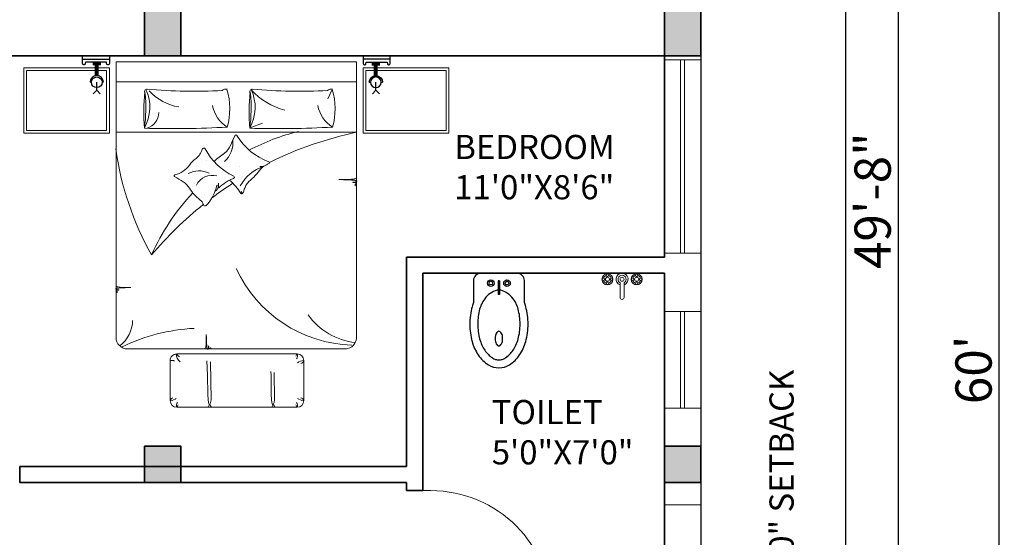
# Model space of a CAD drawing. Units: inches. Extents: x 3321 to 5237, y 11 to 1752.
# Tile 21 of 43: x 4296 to 4541, y 1306 to 1434. Entities that reach past the tile are written whole.
import ezdxf

# ---------------------------------------------------------------- set-up
doc = ezdxf.new("R2010")
doc.units = ezdxf.units.IN
for name, color, linetype, lineweight in [('A-ANNO-DIMS', 2, 'Continuous', 18), ('A-ANNO-TEXT', 7, 'Continuous', 18), ('A-AREA-IDEN', 7, 'Continuous', 18), ('A-COLS', 1, 'Continuous', 35), ('A-DOOR', 4, 'Continuous', 18), ('A-FLOR-EDGE', 7, 'Continuous', 25), ('A-GLAZ', 5, 'Continuous', 18), ('A-WALL', 7, 'Continuous', 35), ('C-PROP', 7, 'Continuous', 30), ('FUR', 42, 'Continuous', 18), ('Сантехника', 7, 'Continuous', 18)]:
    doc.layers.add(name, color=color, linetype=linetype, lineweight=lineweight)
for name, color, linetype in [('CEIL', 4, 'Continuous'), ('ELEC', 4, 'Continuous'), ('SANTEH', 7, 'Continuous'), ('wood', 26, 'Continuous')]:
    doc.layers.add(name, color=color, linetype=linetype)
doc.styles.get("Standard").update_dxf_attribs({"font": 'arial.ttf'})
doc.dimstyles.new('ISO-25', dxfattribs={"dimtxt": 9, "dimasz": 2.5, "dimexe": 1.25, "dimexo": 0.625, "dimtad": 1, "dimdec": 1, "dimlunit": 3, "dimtxsty": 'Standard', "dimcen": 2.5, "dimclrd": 4, "dimclre": 4, "dimclrt": 256, "dimadec": 0, "dimazin": 0, "dimtfac": 1, "dimtdec": 1, "dimtmove": 0, "dimatfit": 3, "dimfxl": 1, "dimarcsym": 0})

# ---------------------------------------------------------------- blocks, each defined once
blk = doc.blocks.new('*U5')
for p, q in [((0, 0), (0, -6)), ((-30, 0), (-30, -6))]:
    blk.add_line(p, q)
blk.add_lwpolyline([(0, 0), (0, 30), (-1.75, 30), (-1.75, 0)], close=True)
blk.add_arc((0, 0), 30, 90, 180)
blk = doc.blocks.new('*D61')
at = {"layer": 'A-ANNO-DIMS', "color": 0, "lineweight": -2, "transparency": 16777216}
for p, q in [((4502.01, 1687.34), (4515.69, 1687.34)), ((4514.44, 1093.84), (4514.44, 1684.84)), ((4502.01, 1091.34), (4515.69, 1091.34))]:
    blk.add_line(p, q, dxfattribs=at)
at = {"layer": 'A-ANNO-DIMS', "color": 0, "transparency": 16777216}
for points in [[(4514.03, 1684.84), (4514.86, 1684.84), (4514.44, 1687.34)], [(4514.03, 1093.84), (4514.86, 1093.84), (4514.44, 1091.34)]]:
    blk.add_solid(points, dxfattribs=at)
at = {"layer": 'Defpoints', "color": 0, "transparency": 16777216}
for p in [(4501.39, 1687.34), (4514.44, 1687.34), (4501.39, 1091.34)]:
    blk.add_point(p, dxfattribs=at)
at = {"layer": 'A-ANNO-DIMS', "color": 0, "transparency": 16777216, "insert": (4509.22, 1389.34), "char_height": 9, "attachment_point": 5, "rotation": 90}
blk.add_mtext('49\'-8"', dxfattribs=at)
blk = doc.blocks.new('*D64')
at = {"layer": 'A-ANNO-DIMS', "color": 0, "lineweight": -2, "transparency": 16777216}
for p, q in [((4502.01, 1707.34), (4540.73, 1707.34)), ((4539.48, 989.84), (4539.48, 1704.84)), ((4502.01, 987.34), (4540.73, 987.34))]:
    blk.add_line(p, q, dxfattribs=at)
at = {"layer": 'A-ANNO-DIMS', "color": 0, "transparency": 16777216}
for points in [[(4539.06, 1704.84), (4539.9, 1704.84), (4539.48, 1707.34)], [(4539.06, 989.84), (4539.9, 989.84), (4539.48, 987.34)]]:
    blk.add_solid(points, dxfattribs=at)
at = {"layer": 'Defpoints', "color": 0, "transparency": 16777216}
for p in [(4501.39, 1707.34), (4539.48, 1707.34), (4501.39, 987.34)]:
    blk.add_point(p, dxfattribs=at)
at = {"layer": 'A-ANNO-DIMS', "color": 0, "transparency": 16777216, "insert": (4534.26, 1347.34), "char_height": 9, "attachment_point": 5, "rotation": 90}
blk.add_mtext("60'", dxfattribs=at)
blk = doc.blocks.new('*X127')
at = {"color": 0}
for p, q in [((3155.9, 8182.9), (3155.9, 8182.9)), ((3147.8, 8143.4), (3147.8, 8143.4)), ((3283, 8049.6), (3283, 8049.6)), ((3209.5, 8023.9), (3209.5, 8023.9)), ((3251.6, 7997), (3251.6, 7997)), ((3154.1, 7950.7), (3154.1, 7950.7))]:
    blk.add_line(p, q, dxfattribs=at)
blk = doc.blocks.new('*X126')
at = {"color": 0}
for p, q in [((3155.9, 8182.9), (3155.9, 8182.9)), ((3139.8, 7939.7), (3139.8, 7939.7))]:
    blk.add_line(p, q, dxfattribs=at)
blk = doc.blocks.new('*X125')
at = {"color": 0}
for p, q in [((3155.9, 8182.9), (3155.9, 8182.9)), ((3139.8, 7939.7), (3139.8, 7939.7))]:
    blk.add_line(p, q, dxfattribs=at)
blk = doc.blocks.new('*X124')
at = {"color": 0}
for p, q in [((3163, 7776.2), (3163, 7776.2)), ((3422.2, 7761.3), (3422.2, 7761.3)), ((3236.2, 7675.7), (3236.2, 7675.7)), ((3244.3, 7698.6), (3244.3, 7698.6)), ((3340.3, 7689.4), (3340.3, 7689.4))]:
    blk.add_line(p, q, dxfattribs=at)
blk = doc.blocks.new('BED1')
for p, q in [((0, -1000), (0, 800)), ((150, 800), (0, 800)), ((150, 800), (150, -1000)), ((2058.7, 800), (150, 800)), ((528, 800), (528, -1000)), ((211.8, 614.9), (277.5, 585.4)), ((2537.2, 404.9), (2237.2, 404.9)), ((2187.2, 354.9), (2187.2, -545.1)), ((2587.2, -545.1), (2587.2, 354.9)), ((2566.3, 178.5), (2565.2, 177.4)), ((2582, 188.1), (2565.4, 174.8)), ((2565.4, 174.8), (2585.7, 165.4)), ((2582, -287.1), (2565.4, -300.5)), ((2566.3, -296.8), (2565.2, -297.9)), ((2565.4, -300.5), (2585.7, -309.9)), ((2237.2, -595.1), (2537.2, -595.1)), ((150, -1000), (0, -1000)), ((150, -1000), (2063.5, -1000))]:
    blk.add_line(p, q)
for points in [[(934, 797.9), (930.9, 797.7), (928.3, 797.4), (926.3, 796.9), (924.9, 796.3), (923.8, 795.6), (923.1, 794.8), (922.7, 793.8), (922.5, 792.7), (922.4, 791.5), (922.5, 790.3), (922.6, 789.2), (922.6, 788.3), (922.6, 787.6), (922.4, 787.3), (922, 787.4), (921.4, 787.9), (920.6, 788.9), (919.5, 790.2), (918.4, 791.6), (917.1, 793.1), (915.9, 794.6), (914.6, 796), (913.3, 797.1), (912.2, 797.9), (911.1, 798.3), (910.1, 798.4), (909.2, 798), (908.3, 797.1), (907.5, 795.8), (906.8, 793.9), (906, 791.4), (905.4, 788.5), (904.8, 785.2), (904.2, 781.7), (903.7, 778.4), (903.2, 775.4), (902.8, 772.9), (902.5, 771.3), (902.3, 770.6), (902.1, 771.2), (902, 772.8), (901.8, 775.2), (901.7, 778.1), (901.5, 781.5), (901.2, 785), (900.8, 788.4), (900.2, 791.5), (899.5, 794.1), (898.6, 796.2), (897.6, 797.9), (896.5, 799.2), (895.3, 800), (894.1, 800.5), (893, 800.7), (891.9, 800.5), (890.9, 800.1), (890, 799), (889.1, 797.1), (888.3, 794), (887.6, 789.3), (886.9, 782.9), (886.2, 774.2), (885.5, 763.1), (884.8, 749.5), (884.2, 734.2), (883.6, 718.3), (883, 702.8), (882.5, 688.8), (882, 677.5), (881.7, 669.8), (881.5, 666.9), (881.3, 669.4), (881.3, 676.7), (881.3, 687.8), (881.2, 701.5), (881.1, 716.8), (880.8, 732.6), (880.2, 748), (879.4, 761.8), (878.3, 773.2), (876.9, 782.2), (875.1, 789.2), (872.9, 794.4), (870.3, 798), (869, 799)], [(2150, -913.5), (2150, 723.2)], [(2327.6, 182.3), (2530, 185.9), (2550.8, 181.9), (2561.7, 179), (2566, 176.7), (2566.9, 174.4), (2566.3, 171.9), (2562, 169.2), (2550.3, 166.5), (2527.7, 163.9), (2490.6, 161.8), (2345.5, 160.2), (2317.8, 158.5)], [(494.7, 3.1), (458.9, 95.3)], [(2149.7, -259.9), (2150, -268.4), (2150.1, -274.1), (2150.1, -278.1), (2150, -281.4), (2149.8, -284), (2149.5, -286.1), (2149.1, -287.8), (2148.7, -289), (2148.1, -289.9), (2147.4, -290.5), (2146.6, -290.8), (2145.6, -291), (2144.6, -291), (2143.6, -291), (2142.7, -290.9), (2141.9, -290.9), (2141.4, -290.9), (2141.1, -291), (2141.2, -291.4), (2141.7, -291.9), (2142.5, -292.6), (2143.5, -293.4), (2144.7, -294.4), (2146, -295.4), (2147.2, -296.5), (2148.4, -297.6), (2149.3, -298.6), (2150, -299.6), (2150.3, -300.5), (2150.4, -301.3), (2150, -302.1), (2149.3, -302.8), (2148.2, -303.5), (2146.6, -304.1), (2144.6, -304.7), (2142.1, -305.2), (2139.3, -305.7), (2136.5, -306.2), (2133.7, -306.6), (2131.2, -307), (2129.2, -307.3), (2127.8, -307.6), (2127.3, -307.8), (2127.7, -308), (2129, -308.1), (2131, -308.2), (2133.5, -308.3), (2136.3, -308.5), (2139.2, -308.7), (2142, -309), (2144.6, -309.5), (2146.8, -310.1), (2148.6, -310.9), (2150, -311.7), (2151, -312.7), (2151.7, -313.6), (2152.1, -314.6), (2152.3, -315.6), (2152.2, -316.5), (2151.8, -317.3), (2150.9, -318.1), (2149.3, -318.8), (2146.7, -319.4), (2142.8, -320), (2137.4, -320.6), (2130.2, -321.2), (2121, -321.8), (2109.7, -322.3), (2096.9, -322.9), (2083.6, -323.4), (2070.7, -323.9), (2059.1, -324.3), (2049.6, -324.7), (2043.2, -325), (2040.8, -325.2), (2042.9, -325.3), (2049, -325.3), (2058.2, -325.3), (2069.6, -325.4), (2082.3, -325.5), (2095.6, -325.8), (2108.4, -326.2), (2119.9, -326.8), (2129.4, -327.8), (2136.9, -329), (2142.7, -330.5), (2147, -332.3), (2150, -334.4), (2150.9, -335.6)], [(2246.5, -294.4), (2530, -289.4), (2550.8, -293.4), (2561.7, -296.3), (2566, -298.6), (2566.9, -300.8), (2566.3, -303.4), (2562, -306.1), (2550.3, -308.8), (2527.7, -311.3), (2490.6, -313.5), (2345.5, -315), (2238.6, -321.8)], [(1733.7, -998.3), (1731.1, -998.1), (1729, -997.8), (1727.4, -997.4), (1726.1, -997), (1725.2, -996.4), (1724.7, -995.7), (1724.3, -994.8), (1724.1, -993.9), (1724.1, -992.9), (1724.1, -991.9), (1724.2, -991), (1724.2, -990.2), (1724.2, -989.7), (1724.1, -989.4), (1723.8, -989.5), (1723.2, -990), (1722.5, -990.8), (1721.7, -991.8), (1720.7, -993), (1719.7, -994.3), (1718.6, -995.5), (1717.5, -996.6), (1716.5, -997.6), (1715.5, -998.3), (1714.6, -998.6), (1713.8, -998.6), (1713, -998.3), (1712.3, -997.6), (1711.7, -996.5), (1711, -994.9), (1710.4, -992.9), (1709.9, -990.4), (1709.4, -987.6), (1708.9, -984.8), (1708.5, -982), (1708.1, -979.5), (1707.8, -977.4), (1707.5, -976.1), (1707.3, -975.5), (1707.1, -976), (1707, -977.3), (1706.9, -979.3), (1706.8, -981.8), (1706.7, -984.6), (1706.4, -987.5), (1706.1, -990.3), (1705.6, -992.9), (1705, -995.1), (1704.2, -996.9), (1703.4, -998.3), (1702.4, -999.3), (1701.5, -1000), (1700.5, -1000.4), (1699.6, -1000.6), (1698.7, -1000.4), (1697.8, -1000.1), (1697, -999.2), (1696.3, -997.6), (1695.7, -995), (1695.1, -991.1), (1694.5, -985.7), (1693.9, -978.5), (1693.3, -969.3), (1692.8, -957.9), (1692.2, -945.2), (1691.7, -931.9), (1691.2, -919), (1690.8, -907.4), (1690.4, -897.9), (1690.1, -891.5), (1689.9, -889.1), (1689.8, -891.2), (1689.8, -897.3), (1689.8, -906.5), (1689.7, -917.9), (1689.6, -930.6), (1689.4, -943.8), (1688.9, -956.6), (1688.3, -968.1), (1687.3, -977.6), (1686.1, -985.2), (1684.6, -991), (1682.8, -995.3), (1680.7, -998.3), (1679.6, -999.2)]]:
    blk.add_lwpolyline(points)
for points in [[(205.5, 619.6, 0.267769), (215.1, 582.4, -0.037739), (204.3, 21.8, 0.684696), (236.7, 5.5, -0.060702), (497.2, 0.1, -0.046649), (225.9, 3.1, -1.318436)], [(489.2, 619.6, 0.144019), (207.6, 617.9, 0.248643)], [(497.2, 0.1, 0.021276), (489.2, 619.6, -0.206383), (326.6, 509.4, 0.237198)], [(211.8, 12.8, 0.143972), (361.6, 262.9, 1.292232)], [(886.4, -150, -0.069098), (985, -66.5, 0.658965), (982.1, -48.7, -0.049789), (927.4, -29, -0.103757), (896.6, -5.4, 0.055725), (800.9, 83.3, -0.11866), (782.7, 104.9, 0.016811), (761.6, 143.9, 0.70791), (748.3, 144, -0.16964), (551.9, -96.6, 0.664036), (554, -110.7, 0.023706), (627, -144.7, -0.134834), (683.2, -188, 0.012748), (746.3, -267.4)], [(969.1, -259.1, 0.263265), (936.3, -236.9, -0.026108), (909.2, -233.2, 0.027613), (945.1, -234.2, -0.089259), (872.7, -120, 0.662242), (857.6, -119.3, -0.162037), (651.8, -332.7, 0.676499), (654, -354.5, -0.160513), (722.9, -401.5, 0.07473), (773.5, -450.3, -0.187721), (845.5, -559.9, 0.70791), (858.8, -561.4, -0.010003), (898.6, -497.3, -0.113819), (947.3, -450.2, 0.099539), (1032.5, -372.4, -0.173425), (1070.9, -346.4, 0.589988), (1076.2, -326.1, 0.137312), (923.9, -245.9, 0.137312)], [(205.5, -168.2, 0.267769), (215.1, -205.4, -0.037739), (204.3, -766, 0.684696), (236.7, -782.3, -0.060702), (497.2, -787.7, -0.046649), (225.9, -784.7, -1.318436)], [(489.2, -168.2, 0.144019), (207.6, -169.9, 0.248643)], [(497.2, -787.7, 0.021276), (489.2, -168.2, -0.206383), (326.6, -278.4, 0.237198)], [(1446, -733.4, -0.095039), (652.8, -1001.7)]]:
    blk.add_lwpolyline(points, format="xyb")
for centre, radius, start, end in [((3208.8, 1363.3), 2739.4, 191.86791, 206.32469), ((1138.6, 793.9), 983.2, 294.60777, 358.30329), ((1608.1, 842.5), 496.3, 305.19014, 354.02057), ((2062.7, 713.7), 86.5, 0, 93.53765), ((2237.2, 354.9), 50, 90, 180), ((2321.1, 409.7), 84.5, 185.61958, 217.13957), ((2227.5, 373.5), 32.8, 17.83305, 72.80048), ((2546.9, 373.5), 32.8, 107.19952, 162.16695), ((2453.3, 409.7), 84.5, 322.86043, 354.38042), ((2537.2, 354.9), 50, 0, 90), ((2098.7, 754.7), 1625, 193.90497, 207.81692), ((2201.9, 323.3), 34.8, 50.8413, 114.9586), ((2212.2, 381.5), 36.5, 226.80948, 258.3841), ((2572.5, 323.3), 34.8, 65.0414, 129.1587), ((2562.2, 381.5), 36.5, 281.6159, 313.19052), ((751.8, 88.7), 34.9, 336.83517, 27.72181), ((684.2, 86), 100.3, 353.675, 10.88198), ((1074.1, 198.8), 306.1, 197.86019, 241.51221), ((341.4, -277.7), 318.5, 60.71255, 115.00895), ((983.7, -79.5), 20.8, 73.79673, 130.45661), ((978.5, -68.6), 14.3, 39.7097, 85.9506), ((602.5, -324), 198.6, 43.20348, 95.05559), ((3208.8, 1363.3), 2739.4, 212.93136, 216.95099), ((981.1, -281.8), 131.1, 164.0372, 243.45361), ((980, -379), 163.4, 152.61037, 209.36102), ((3208.8, 1363.3), 2739.4, 218.63292, 229.94485), ((2098.7, 754.7), 1625, 226.58872, 246.3156), ((3402.5, -342.9), 1408.5, 182.99169, 205.68187), ((-34.4, -471.2), 376.5, 312.01178, 350.96348), ((2178, -513.5), 33, 286.18268, 338.13858), ((2237.2, -545.1), 50, 180, 270), ((2188.1, -476.2), 73, 269.45125, 322.80265), ((2271.1, -580.9), 35.8, 148.90546, 197.55407), ((2546.9, -563.8), 32.8, 197.83305, 252.80048), ((2453.3, -600), 84.5, 5.61958, 37.13957), ((2537.2, -545.1), 50, 270, 0), ((2572.5, -513.6), 34.8, 230.8413, 294.9586), ((2562.2, -571.8), 36.5, 46.80948, 78.3841), ((375.7, -807.4), 128.2, 17.40732, 88.51286), ((341.4, -1065.5), 318.5, 60.71255, 115.00895), ((1929.1, -1126), 250.5, 37.85533, 88.44053), ((2063.5, -913.5), 86.5, 270, 0)]:
    blk.add_arc(centre, radius, start, end)
for name in ['*X126', '*X125', '*X127', '*X124']:
    blk.add_blockref(name, (-2425.3, -8101.4))
blk = doc.blocks.new('APLIQ')
at = {"layer": 'ELEC'}
for p, q in [((0, 0.2), (-0.0261, 0.2261)), ((0, 0.2), (0.0261, 0.2261)), ((0, 0.2), (0, 0.14)), ((-0.05, 0.14), (-0.04, 0.14)), ((-0.01, 0.09), (-0.01, 0.01)), ((0, 0.09), (0, 0)), ((0.01, 0.09), (0.01, 0.01)), ((0.04, 0.14), (0.05, 0.14)), ((-0.03, 0.01), (0.03, 0.01)), ((-0.03, 0), (0.03, 0))]:
    blk.add_line(p, q, dxfattribs=at)
blk.add_circle((0, 0.14), 0.04, dxfattribs=at)
blk.add_arc((0, 0.14), 0.05, 180, 0, dxfattribs=at)
blk = doc.blocks.new('A$C68AE1801')
at = {"layer": 'FUR'}
for points in [[(2.5416, 3.18), (2.5416, 2.54), (2.0516, 2.54), (2.0516, 3.18)], [(2.5216, 3.16), (2.5216, 2.56), (2.0716, 2.56), (2.0716, 3.16)], [(2.5416, 0), (2.5416, 0.64), (2.0516, 0.64), (2.0516, 0)], [(2.5216, 0.02), (2.5216, 0.62), (2.0716, 0.62), (2.0716, 0.02)]]:
    blk.add_lwpolyline(points, close=True, dxfattribs=at)
at = {"layer": 'wood'}
for p, q in [((2.6057, 2.74), (2.6057, 2.54)), ((2.6057, 0.44), (2.6057, 0.64))]:
    blk.add_line(p, q, dxfattribs=at)
for points in [[(2.5657, 2.728), (2.5657, 2.732, -0.414214), (2.5737, 2.74), (2.6321, 2.74), (2.6321, 2.54), (2.5737, 2.54, -0.414214), (2.5657, 2.548), (2.5657, 2.552, -0.414214), (2.5737, 2.56), (2.5777, 2.56, 0.414214), (2.5857, 2.568), (2.5857, 2.712, 0.414214), (2.5777, 2.72), (2.5737, 2.72, -0.414214)], [(2.5657, 0.452), (2.5657, 0.448, 0.414214), (2.5737, 0.44), (2.6321, 0.44), (2.6321, 0.64), (2.5737, 0.64, 0.414214), (2.5657, 0.632), (2.5657, 0.628, 0.414214), (2.5737, 0.62), (2.5777, 0.62, -0.414214), (2.5857, 0.612), (2.5857, 0.468, -0.414214), (2.5777, 0.46), (2.5737, 0.46, 0.414214)]]:
    blk.add_lwpolyline(points, format="xyb", close=True, dxfattribs=at)
at = {"layer": 'CEIL', "rotation": 90}
blk.add_blockref('APLIQ', (2.5736, 2.634), dxfattribs=at)
at = {"layer": 'CEIL', "xscale": -1, "rotation": 90}
blk.add_blockref('APLIQ', (2.5736, 0.546), dxfattribs=at)
at = {"layer": 'FUR', "xscale": 0.001, "yscale": 0.001, "zscale": 0.001, "rotation": 180}
blk.add_blockref('BED1', (2.5872, 1.49), dxfattribs=at)
blk = doc.blocks.new('K10-45')
at = {"layer": 'SANTEH'}
for p, q in [((-18.9, 83.4), (-18.9, 177.1)), ((-18.9, 177.1), (-8.9, 177.1)), ((-8.9, 83.4), (-8.9, 177.1)), ((-18.9, 83.4), (-8.9, 83.4))]:
    blk.add_line(p, q, dxfattribs=at)
for points in [[(160.3, 230.4, 0.023928), (169.9, 259.6, 0.067459), (186.1, 379, 0.067459), (169.9, 498.4, 0.079812), (127.5, 591.1, 0.107118), (58, 658.5, 0.139889), (-13.9, 679, 0.139889), (-85.8, 658.5, 0.107118), (-155.3, 591.1, 0.079812), (-197.7, 498.4, 0.067459), (-213.9, 379, 0.067459), (-197.7, 259.6, 0.023928), (-188.1, 230.4), (-188.1, 80.2, 0.414214), (-138.1, 30.2), (110.3, 30.2, 0.414214), (160.3, 80.2)], [(-39.4, 478.5, 0.052061), (-37.3, 458.3, 0.065919), (-32, 443.1, 0.104629), (-22.6, 431.5, 0.172287), (-13.9, 428.4, 0.172287), (-5.2, 431.5, 0.104629), (4.1, 443.1, 0.065919), (9.5, 458.3, 0.052061), (11.6, 478.5, 0.052061), (9.5, 498.7, 0.065919), (4.1, 513.9, 0.104629), (-5.2, 525.5, 0.172287), (-13.9, 528.6, 0.172287), (-22.6, 525.5, 0.104629), (-32, 513.9, 0.065919), (-37.3, 498.7, 0.052061)]]:
    blk.add_lwpolyline(points, format="xyb", close=True, dxfattribs=at)
blk.add_lwpolyline([(-3.9, 147), (-1.4, 147.2), (10.9, 150.3), (23, 155.1), (34.7, 161.4), (45.9, 168.8), (56.5, 177.2), (66.3, 186.2), (75.2, 195.5), (83.2, 205), (90.3, 214.7), (96.5, 224.5), (102, 234.5), (106.9, 244.7), (111.1, 255.3), (114.8, 266.2), (118.1, 277.6), (121.1, 289.3), (123.7, 301.4), (126, 313.8), (127.9, 326.5), (129.3, 339.5), (130.4, 352.6), (131.1, 365.8), (131.3, 379), (131.1, 392.2), (130.4, 405.4), (129.3, 418.5), (127.9, 431.4), (126, 444.2), (123.7, 456.6), (121.1, 468.7), (118.1, 480.4), (114.8, 491.7), (111.2, 502.6), (107.3, 513.1), (103, 523.1), (98.4, 532.7), (93.5, 541.9), (88.3, 550.7), (82.8, 559.1), (77.1, 567.1), (71, 574.6), (64.9, 581.7), (58.5, 588.3), (52.1, 594.4), (45.7, 600), (39.3, 605), (33, 609.4), (26.9, 613.2), (20.8, 616.4), (14.9, 619), (9, 621.1), (3.2, 622.7), (-2.5, 623.8), (-8.2, 624.5), (-13.9, 624.7), (-19.6, 624.5), (-25.3, 623.8), (-31, 622.7), (-36.8, 621.1), (-42.7, 619), (-48.6, 616.4), (-54.7, 613.2), (-60.9, 609.4), (-67.2, 605), (-73.5, 600), (-80, 594.4), (-86.4, 588.3), (-92.7, 581.7), (-98.9, 574.6), (-104.9, 567.1), (-110.6, 559.1), (-116.1, 550.7), (-121.3, 541.9), (-126.2, 532.7), (-130.8, 523.1), (-135.1, 513.1), (-139, 502.6), (-142.7, 491.7), (-146, 480.4), (-148.9, 468.7), (-151.5, 456.6), (-153.8, 444.2), (-155.7, 431.4), (-157.2, 418.5), (-158.2, 405.4), (-158.9, 392.2), (-159.1, 379), (-158.9, 365.8), (-158.2, 352.6), (-157.2, 339.5), (-155.7, 326.5), (-153.8, 313.8), (-151.5, 301.4), (-148.9, 289.3), (-146, 277.6), (-142.6, 266.2), (-138.9, 255.3), (-134.7, 244.7), (-129.8, 234.5), (-124.4, 224.5), (-118.1, 214.7), (-111, 205), (-103.1, 195.5), (-94.1, 186.2), (-84.3, 177.2), (-73.7, 168.8), (-62.5, 161.4), (-50.8, 155.1), (-38.7, 150.3), (-26.4, 147.2), (-23.9, 147)], dxfattribs=at)
for centre, radius in [((-69.2, 98.1), 22.4), ((-69.2, 98.1), 12.4), ((41.4, 98.1), 22.4), ((41.4, 98.1), 12.4)]:
    blk.add_circle(centre, radius, dxfattribs=at)
blk = doc.blocks.new('Faucet - Bathroom top')
for p, q in [((-4.107, 0.125), (-4.375, 0.125)), ((-3.75, 0.4788), (-3.75, 0.75)), ((-3.5, 0.482), (-3.5, 0.75)), ((-3.1461, 0.125), (-2.875, 0.125)), ((3.143, 0.125), (2.875, 0.125)), ((3.5, 0.4788), (3.5, 0.75)), ((3.75, 0.482), (3.75, 0.75)), ((4.1039, 0.125), (4.375, 0.125)), ((-4.1039, -0.125), (-4.375, -0.125)), ((-3.75, -0.4821), (-3.75, -0.75)), ((-3.5, -0.4789), (-3.5, -0.75)), ((-3.143, -0.125), (-2.875, -0.125)), ((-0.5, -0.8639), (-0.5, -4.5)), ((0.5, -4.5), (0.5, -0.8631)), ((3.1461, -0.125), (2.875, -0.125)), ((3.5, -0.4821), (3.5, -0.75)), ((3.75, -0.4789), (3.75, -0.75)), ((4.107, -0.125), (4.375, -0.125))]:
    blk.add_line(p, q)
for centre, radius in [((-3.625, 0), 1.375), ((-4.625, 0), 0.2795), ((-3.625, 0), 0.5), ((-3.625, 1), 0.2795), ((-2.625, 0), 0.2795), ((0, 0), 0.5), ((3.625, 0), 1.375), ((2.625, 0), 0.2795), ((3.625, 0), 0.5), ((3.625, 1), 0.2795), ((4.625, 0), 0.2795), ((-3.625, -1), 0.2795), ((3.625, -1), 0.2795)]:
    blk.add_circle(centre, radius)
for centre, radius, start, end in [((-3.625, 0), 1, 105.2407, 164.2093), ((-3.625, 0), 1, 16.44125, 74.07887), ((0, 0), 1.5, 289.6514, 250.3603), ((0, 0), 1, 300.3431, 239.7554), ((3.625, 0), 1, 106.12, 164.0884), ((3.625, 0), 1, 16.23422, 73.90469), ((-3.625, 0), 1, 196.2342, 253.9047), ((-3.625, 0), 1, 286.12, 344.0884), ((3.625, 0), 1, 196.4413, 254.0789), ((3.625, 0), 1, 285.2407, 344.2093), ((0, -4.5), 0.5, 180, 0)]:
    blk.add_arc(centre, radius, start, end)
blk = doc.blocks.new('COL-9X18-IN')
h = blk.add_hatch(color=256)
h.dxf.hatch_style = 1
h.paths.add_polyline_path([(9, 18), (0, 18), (0, 0), (9, 0)])
blk.add_lwpolyline([(0, 0), (9, 0), (9, 18), (0, 18)], close=True)
blk = doc.blocks.new('COL-9X12-FURN-PLAN')
h = blk.add_hatch(color=256)
h.dxf.hatch_style = 1
h.paths.add_polyline_path([(0, 12), (0, 0), (9, 0), (9, 12)])
blk.add_lwpolyline([(0, 0), (9, 0), (9, 12), (0, 12)], close=True)
blk = doc.blocks.new('COL-9X9-FURN-PLAN')
h = blk.add_hatch(color=256)
h.dxf.hatch_style = 1
h.paths.add_polyline_path([(9, 9), (0, 9), (0, 0), (9, 0)])
blk.add_lwpolyline([(0, 0), (9, 0), (9, 9), (0, 9)], close=True)
blk = doc.blocks.new('WIN-48IN-9IN-WALL')
for p, q in [((0, 0), (0, 9)), ((48, 0), (48, 9)), ((0, 5), (48, 5)), ((0, 4), (48, 4))]:
    blk.add_line(p, q)
blk = doc.blocks.new('WIN-24IN-9IN-WALL')
for p, q in [((9, 24), (0, 24)), ((4, 24), (4, 0)), ((5, 24), (5, 0)), ((9, 0), (0, 0))]:
    blk.add_line(p, q)
blk = doc.blocks.new('PROPERTY-40X60FT')
blk.add_line((0, 720), (0, 0))

msp = doc.modelspace()

# ---------------------------------------------------------------- linework, layer by layer
at = {"layer": 'A-FLOR-EDGE'}
msp.add_line((4465.39, 1687.34), (4465.39, 1091.34), dxfattribs=at)
at = {"layer": 'A-GLAZ'}
msp.add_line((4465.39, 1313.84), (4456.39, 1313.84), dxfattribs=at)
at = {"layer": 'A-WALL'}
for p, q in [((4260.39, 1425.34), (4327.39, 1425.34)), ((4336.39, 1425.34), (4456.39, 1425.34)), ((4456.39, 1425.34), (4456.39, 1375.34)), ((4392.39, 1375.34), (4392.39, 1323.34)), ((4392.39, 1375.34), (4456.39, 1375.34)), ((4396.39, 1371.34), (4396.39, 1317.34)), ((4396.39, 1371.34), (4456.39, 1371.34)), ((4456.39, 1371.34), (4456.39, 1287.34)), ((4296.39, 1323.34), (4392.39, 1323.34)), ((4296.39, 1323.34), (4296.39, 1319.34)), ((4296.39, 1319.34), (4392.39, 1319.34)), ((4392.39, 1319.34), (4392.39, 1317.34)), ((4392.39, 1317.34), (4396.39, 1317.34))]:
    msp.add_line(p, q, dxfattribs=at)

# ---------------------------------------------------------------- block references
at = {"layer": 'A-COLS', "rotation": 180}
msp.add_blockref('COL-9X18-IN', (4336.39, 1443.34), dxfattribs=at)
at = {"layer": 'A-COLS'}
for name, p in [('COL-9X12-FURN-PLAN', (4456.39, 1425.34)), ('COL-9X9-FURN-PLAN', (4327.39, 1319.34)), ('COL-9X9-FURN-PLAN', (4456.39, 1319.34))]:
    msp.add_blockref(name, p, dxfattribs=at)
at = {"layer": 'A-DOOR', "rotation": 270}
msp.add_blockref('*U5', (4398.39, 1287.34), dxfattribs=at)
at = {"layer": 'A-GLAZ', "rotation": 89.99999999999812}
msp.add_blockref('WIN-48IN-9IN-WALL', (4465.39, 1376.34), dxfattribs=at)
at = {"layer": 'A-GLAZ'}
msp.add_blockref('WIN-24IN-9IN-WALL', (4456.39, 1337.84), dxfattribs=at)
at = {"layer": 'C-PROP', "rotation": 180}
msp.add_blockref('PROPERTY-40X60FT', (4501.39, 1707.34), dxfattribs=at)
at = {"layer": 'FUR', "xscale": 33.17188472218209, "yscale": 33.17188472218209, "zscale": 33.17188472218209, "rotation": 90}
msp.add_blockref('A$C68AE1801', (4402.89, 1338.03), dxfattribs=at)
at = {"layer": 'Сантехника', "xscale": 0.0362080263207385, "yscale": 0.0362080263207385, "zscale": 0.0362080263207385, "rotation": 180}
msp.add_blockref('K10-45', (4414.81, 1372.43), dxfattribs=at)
at = {"layer": 'Сантехника', "xscale": -1}
msp.add_blockref('Faucet - Bathroom top', (4445.87, 1369.84), dxfattribs=at)

# ---------------------------------------------------------------- texts
at = {"layer": 'A-ANNO-TEXT', "insert": (4482.45, 1294.84), "char_height": 6, "attachment_point": 1, "rotation": 90}
msp.add_mtext_dynamic_manual_height_columns('3\'0" SETBACK', width=97.3114, gutter_width=25, heights=[0], dxfattribs=at)
at = {"layer": 'A-AREA-IDEN', "char_height": 6, "attachment_point": 1}
for s, insert in [('BEDROOM\\P11\'0"X8\'6"', (4404.22, 1405.7)), ('TOILET\\P5\'0"X7\'0"', (4413.53, 1339.85))]:
    msp.add_mtext_dynamic_manual_height_columns(s, width=97.3114, gutter_width=25, heights=[0], dxfattribs=dict(at, insert=insert))

# ---------------------------------------------------------------- dimensions: what is measured, and where the dimension line sits
at = {"layer": 'A-ANNO-DIMS'}
for base, p1, p2, angle, override, picture, middle in [((4539.48, 1707.34), (4501.39, 987.34), (4501.39, 1707.34), 270, {"dimclrd": 0, "dimclre": 0, "dimclrt": 0}, '*D64', (4534.26, 1347.34)), ((4514.44, 1687.34), (4501.39, 1091.34), (4501.39, 1687.34), 90, {"dimclrd": 0, "dimclre": 0, "dimclrt": 0, "dimtmove": 1}, '*D61', (4509.22, 1389.34))]:
    dim = msp.add_linear_dim(base=base, p1=p1, p2=p2, angle=angle, dimstyle='ISO-25', override=override, dxfattribs=at)
    dim.commit()
    dim.dimension.update_dxf_attribs({"geometry": picture, "text_midpoint": middle})

doc.saveas('drawing.dxf')
